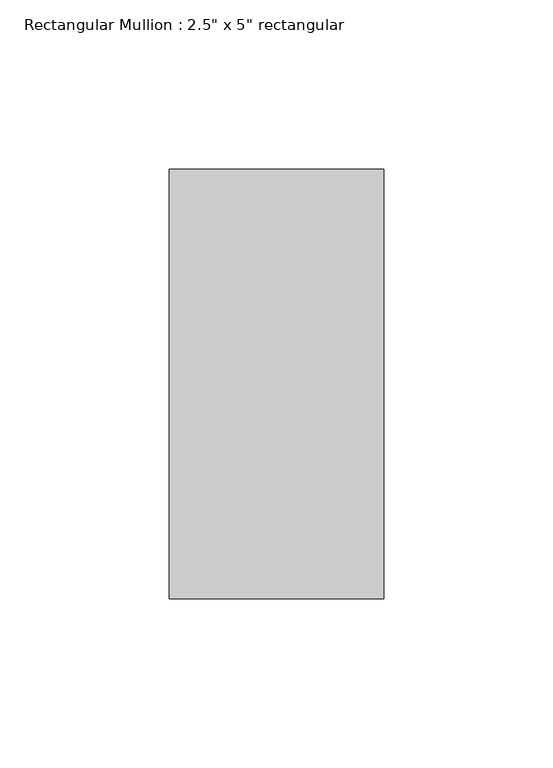
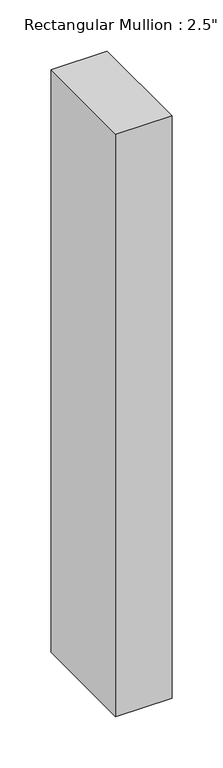
"""IFC4 building model written with IfcOpenShell, lengths in millimetres: member geometry."""

from ifc_helpers import new_model, si_unit, frame, origin, place, context, project, spatial, polyline, outline, extrude, source, transform, mapped, element, save


def member_a9816f27(model_context):
    return source(origin(), model_context, "Body", "SweptSolid", [
        extrude(outline(polyline([(0.0, 63.5), (0.0, -63.5), (-63.5, -63.5), (-63.5, 63.5), (0.0, 63.5)])), frame((0.0, 0.0, -696.5738172), z_axis=(0.0, 0.0, 1.0), x_axis=(1.0, 0.0, 0.0)), (0.0, 0.0, 1.0), 696.5738172),
    ])


if __name__ == "__main__":
    model = new_model("IFC4")
    model_context = context("Model", 3, world=origin())
    ifc_project = project(units=[si_unit("LENGTHUNIT", "METRE", prefix="MILLI")], contexts=[model_context])
    site = spatial("IfcSite", under=ifc_project)
    building = spatial("IfcBuilding", under=site)
    placement = place(None, origin())
    member_shape = member_a9816f27(model_context)
    element("IfcMember", 1, ObjectType="Rectangular Mullion : 2.5\" x 5\" rectangular", at=placement, inside=building, context=model_context, shape_type="MappedRepresentation", body=[
        mapped(member_shape, transform((0.0, 0.0, 0.0), x_axis=(1.0, 0.0, 0.0), y_axis=(0.0, 1.0, 0.0), z_axis=(0.0, 0.0, 1.0))),
    ])
    save(model, "model.ifc")

# Revit data of these elements
# Type "Rectangular Mullion : 2.5\" x 5\" rectangular"
#   built-in parameter 1007304 = 0.416667 (stored number, unit not read)
#   built-in parameter 1007301 = 0.104167 (stored number, unit not read)
#   built-in parameter 1007300 = 0.104167 (stored number, unit not read)
# Element 1 (IfcMember, "Rectangular Mullion : 2.5\" x 5\" rectangular")
#   Materials on its faces: "Aluminum"
# Materials
#   "Aluminum": class "Metal", colour RGB 247 247 247, transparency 0, Description = "Aluminum 6061", Cost = 0
